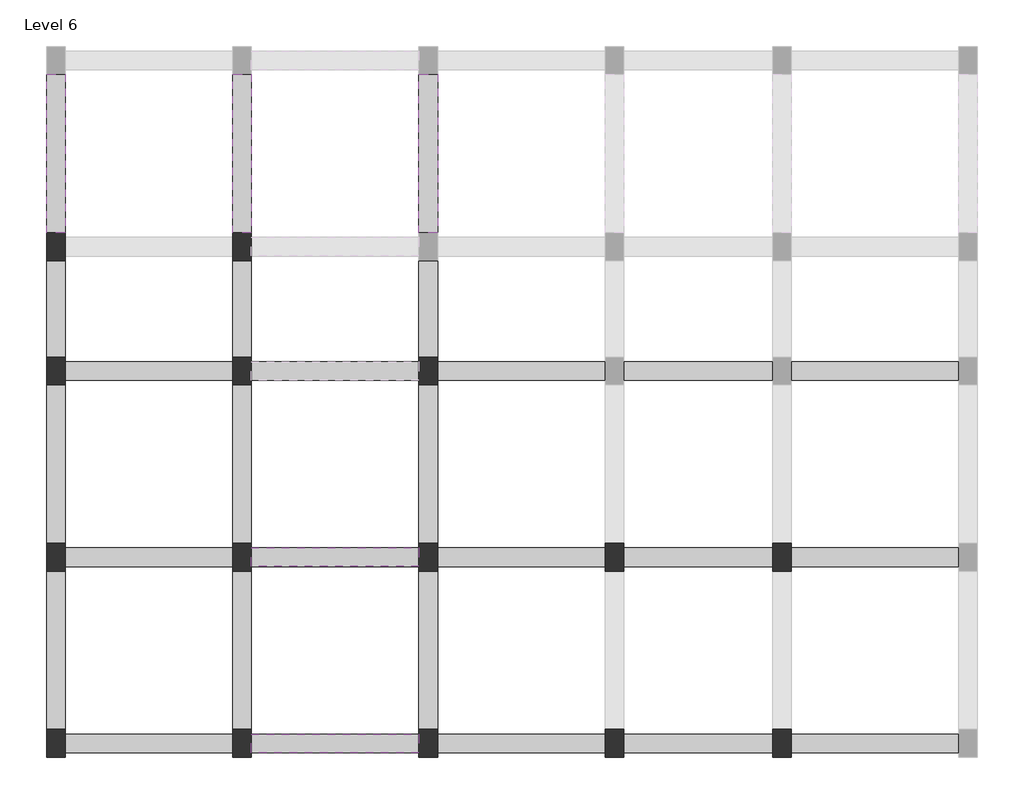
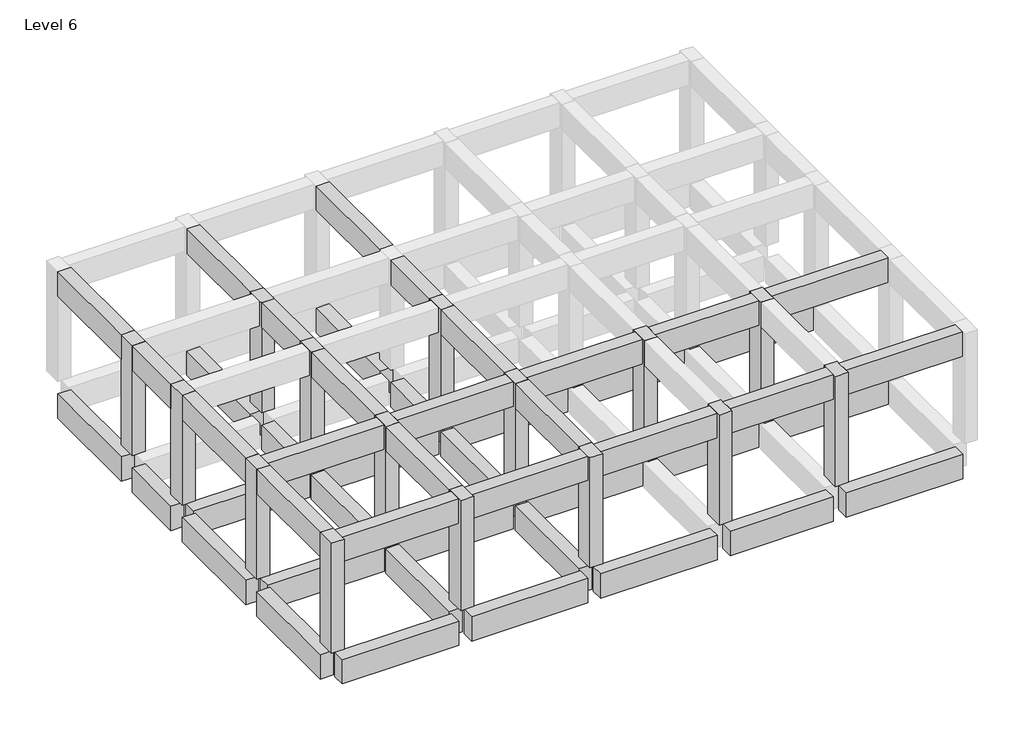
# One storey, part 1 of 2: 15 columns, 11 beams.
"""IFC4 building model written with IfcOpenShell, lengths in millimetres."""

from ifc_helpers import new_model, si_unit, frame, origin, place, context, project, spatial, polyline, outline, extrude, faceted_brep, element, save

model = new_model("IFC4")

# Units and contexts
model_context = context("Model", 3, world=origin())
ifc_project = project(units=[si_unit("LENGTHUNIT", "METRE", prefix="MILLI")], contexts=[model_context])

# Site, building, storey
site = spatial("IfcSite", under=ifc_project)
building = spatial("IfcBuilding", under=site)
storey = spatial("IfcBuildingStorey", under=building, Name="Level 6", Elevation=15240.0)

# Beams
placement = place(None, origin())
element("IfcBeam", 1, ObjectType="Concrete-Rectangular Beam : 12 x 24", at=placement, inside=storey, context=model_context, shape_type="SweptSolid", body=[
    extrude(outline(polyline([(2607.7603583, 7596.6647757), (2607.7603583, 7291.8647757), (-135.4396417, 7291.8647757), (-135.4396417, 7596.6647757), (2607.7603583, 7596.6647757)])), frame((0.0, 0.0, 14325.6), z_axis=(0.0, 0.0, 1.0), x_axis=(1.0, 0.0, 0.0)), (0.0, 0.0, 1.0), 609.6),
    extrude(outline(polyline([(-12022.6396417, 7291.8647757), (-12022.6396417, 7596.6647757), (-9279.4396417, 7596.6647757), (-9279.4396417, 7291.8647757), (-12022.6396417, 7291.8647757)])), frame((0.0, 0.0, 14325.6), z_axis=(0.0, 0.0, 1.0), x_axis=(1.0, 0.0, 0.0)), (0.0, 0.0, 1.0), 609.6),
    extrude(outline(polyline([(-8974.6396417, 7291.8647757), (-8974.6396417, 7596.6647757), (-6231.4396417, 7596.6647757), (-6231.4396417, 7291.8647757), (-8974.6396417, 7291.8647757)])), frame((0.0, 0.0, 14325.6), z_axis=(0.0, 0.0, 1.0), x_axis=(1.0, 0.0, 0.0)), (0.0, 0.0, 1.0), 609.6),
    extrude(outline(polyline([(-5926.6396417, 7291.8647757), (-5926.6396417, 7596.6647757), (-3183.4396417, 7596.6647757), (-3183.4396417, 7291.8647757), (-5926.6396417, 7291.8647757)])), frame((0.0, 0.0, 14325.6), z_axis=(0.0, 0.0, 1.0), x_axis=(1.0, 0.0, 0.0)), (0.0, 0.0, 1.0), 609.6),
    extrude(outline(polyline([(-2878.6396417, 7291.8647757), (-2878.6396417, 7596.6647757), (-440.2396417, 7596.6647757), (-440.2396417, 7291.8647757), (-2878.6396417, 7291.8647757)])), frame((0.0, 0.0, 14325.6), z_axis=(0.0, 0.0, 1.0), x_axis=(1.0, 0.0, 0.0)), (0.0, 0.0, 1.0), 609.6),
])
element("IfcBeam", 2, ObjectType="Concrete-Rectangular Beam : 12 x 24", at=placement, inside=storey, context=model_context, shape_type="SweptSolid", body=[
    extrude(outline(polyline([(2607.7603583, 10644.6647757), (2607.7603583, 10339.8647757), (-135.4396417, 10339.8647757), (-135.4396417, 10644.6647757), (2607.7603583, 10644.6647757)])), frame((0.0, 0.0, 14325.6), z_axis=(0.0, 0.0, 1.0), x_axis=(1.0, 0.0, 0.0)), (0.0, 0.0, 1.0), 609.6),
    extrude(outline(polyline([(-12022.6396417, 10339.8647757), (-12022.6396417, 10644.6647757), (-9279.4396417, 10644.6647757), (-9279.4396417, 10339.8647757), (-12022.6396417, 10339.8647757)])), frame((0.0, 0.0, 14325.6), z_axis=(0.0, 0.0, 1.0), x_axis=(1.0, 0.0, 0.0)), (0.0, 0.0, 1.0), 609.6),
    extrude(outline(polyline([(-8974.6396417, 10339.8647757), (-8974.6396417, 10644.6647757), (-6231.4396417, 10644.6647757), (-6231.4396417, 10339.8647757), (-8974.6396417, 10339.8647757)])), frame((0.0, 0.0, 14325.6), z_axis=(0.0, 0.0, 1.0), x_axis=(1.0, 0.0, 0.0)), (0.0, 0.0, 1.0), 609.6),
    extrude(outline(polyline([(-5926.6396417, 10339.8647757), (-5926.6396417, 10644.6647757), (-3183.4396417, 10644.6647757), (-3183.4396417, 10339.8647757), (-5926.6396417, 10339.8647757)])), frame((0.0, 0.0, 14325.6), z_axis=(0.0, 0.0, 1.0), x_axis=(1.0, 0.0, 0.0)), (0.0, 0.0, 1.0), 609.6),
    extrude(outline(polyline([(-2878.6396417, 10339.8647757), (-2878.6396417, 10644.6647757), (-440.2396417, 10644.6647757), (-440.2396417, 10339.8647757), (-2878.6396417, 10339.8647757)])), frame((0.0, 0.0, 14325.6), z_axis=(0.0, 0.0, 1.0), x_axis=(1.0, 0.0, 0.0)), (0.0, 0.0, 1.0), 609.6),
])
element("IfcBeam", 3, ObjectType="Concrete-Rectangular Beam : 12 x 24", at=placement, inside=storey, context=model_context, shape_type="SweptSolid", body=[
    extrude(outline(polyline([(2607.7603583, 13692.6647757), (2607.7603583, 13387.8647757), (-135.4396417, 13387.8647757), (-135.4396417, 13692.6647757), (2607.7603583, 13692.6647757)])), frame((0.0, 0.0, 14325.6), z_axis=(0.0, 0.0, 1.0), x_axis=(1.0, 0.0, 0.0)), (0.0, 0.0, 1.0), 609.6),
    extrude(outline(polyline([(-12022.6396417, 13387.8647757), (-12022.6396417, 13692.6647757), (-9279.4396417, 13692.6647757), (-9279.4396417, 13387.8647757), (-12022.6396417, 13387.8647757)])), frame((0.0, 0.0, 14325.6), z_axis=(0.0, 0.0, 1.0), x_axis=(1.0, 0.0, 0.0)), (0.0, 0.0, 1.0), 609.6),
    extrude(outline(polyline([(-8974.6396417, 13387.8647757), (-8974.6396417, 13692.6647757), (-6231.4396417, 13692.6647757), (-6231.4396417, 13387.8647757), (-8974.6396417, 13387.8647757)])), frame((0.0, 0.0, 14325.6), z_axis=(0.0, 0.0, 1.0), x_axis=(1.0, 0.0, 0.0)), (0.0, 0.0, 1.0), 609.6),
    extrude(outline(polyline([(-5926.6396417, 13387.8647757), (-5926.6396417, 13692.6647757), (-3183.4396417, 13692.6647757), (-3183.4396417, 13387.8647757), (-5926.6396417, 13387.8647757)])), frame((0.0, 0.0, 14325.6), z_axis=(0.0, 0.0, 1.0), x_axis=(1.0, 0.0, 0.0)), (0.0, 0.0, 1.0), 609.6),
    extrude(outline(polyline([(-2878.6396417, 13387.8647757), (-2878.6396417, 13692.6647757), (-440.2396417, 13692.6647757), (-440.2396417, 13387.8647757), (-2878.6396417, 13387.8647757)])), frame((0.0, 0.0, 14325.6), z_axis=(0.0, 0.0, 1.0), x_axis=(1.0, 0.0, 0.0)), (0.0, 0.0, 1.0), 609.6),
])
element("IfcBeam", 4, ObjectType="Concrete-Rectangular Beam : 12 x 24", at=placement, inside=storey, context=model_context, shape_type="SweptSolid", body=[
    extrude(outline(polyline([(-12022.6396417, 7672.8647757), (-12327.4396417, 7672.8647757), (-12327.4396417, 10263.6647757), (-12022.6396417, 10263.6647757), (-12022.6396417, 7672.8647757)])), frame((0.0, 0.0, 14325.6), z_axis=(0.0, 0.0, 1.0), x_axis=(1.0, 0.0, 0.0)), (0.0, 0.0, 1.0), 609.6),
    extrude(outline(polyline([(-12327.4396417, 18394.9119241), (-12022.6396417, 18394.9119241), (-12022.6396417, 15804.1119241), (-12327.4396417, 15804.1119241), (-12327.4396417, 18394.9119241)])), frame((0.0, 0.0, 14325.6), z_axis=(0.0, 0.0, 1.0), x_axis=(1.0, 0.0, 0.0)), (0.0, 0.0, 1.0), 609.6),
    extrude(outline(polyline([(-12022.6396417, 10720.8647757), (-12327.4396417, 10720.8647757), (-12327.4396417, 13311.6647757), (-12022.6396417, 13311.6647757), (-12022.6396417, 10720.8647757)])), frame((0.0, 0.0, 14325.6), z_axis=(0.0, 0.0, 1.0), x_axis=(1.0, 0.0, 0.0)), (0.0, 0.0, 1.0), 609.6),
    extrude(outline(polyline([(-12022.6396417, 13768.8647757), (-12327.4396417, 13768.8647757), (-12327.4396417, 15346.9119241), (-12022.6396417, 15346.9119241), (-12022.6396417, 13768.8647757)])), frame((0.0, 0.0, 14325.6), z_axis=(0.0, 0.0, 1.0), x_axis=(1.0, 0.0, 0.0)), (0.0, 0.0, 1.0), 609.6),
])
element("IfcBeam", 5, ObjectType="Concrete-Rectangular Beam : 12 x 24", at=placement, inside=storey, context=model_context, shape_type="SweptSolid", body=[
    extrude(outline(polyline([(-8974.6396417, 7672.8647757), (-9279.4396417, 7672.8647757), (-9279.4396417, 10263.6647757), (-8974.6396417, 10263.6647757), (-8974.6396417, 7672.8647757)])), frame((0.0, 0.0, 14325.6), z_axis=(0.0, 0.0, 1.0), x_axis=(1.0, 0.0, 0.0)), (0.0, 0.0, 1.0), 609.6),
    extrude(outline(polyline([(-9279.4396417, 18394.9119241), (-8974.6396417, 18394.9119241), (-8974.6396417, 15804.1119241), (-9279.4396417, 15804.1119241), (-9279.4396417, 18394.9119241)])), frame((0.0, 0.0, 14325.6), z_axis=(0.0, 0.0, 1.0), x_axis=(1.0, 0.0, 0.0)), (0.0, 0.0, 1.0), 609.6),
    extrude(outline(polyline([(-8974.6396417, 10720.8647757), (-9279.4396417, 10720.8647757), (-9279.4396417, 13311.6647757), (-8974.6396417, 13311.6647757), (-8974.6396417, 10720.8647757)])), frame((0.0, 0.0, 14325.6), z_axis=(0.0, 0.0, 1.0), x_axis=(1.0, 0.0, 0.0)), (0.0, 0.0, 1.0), 609.6),
    extrude(outline(polyline([(-8974.6396417, 13768.8647757), (-9279.4396417, 13768.8647757), (-9279.4396417, 15346.9119241), (-8974.6396417, 15346.9119241), (-8974.6396417, 13768.8647757)])), frame((0.0, 0.0, 14325.6), z_axis=(0.0, 0.0, 1.0), x_axis=(1.0, 0.0, 0.0)), (0.0, 0.0, 1.0), 609.6),
])
element("IfcBeam", 6, ObjectType="Concrete-Rectangular Beam : 12 x 24", at=placement, inside=storey, context=model_context, shape_type="SweptSolid", body=[
    extrude(outline(polyline([(-5926.6396417, 7672.8647757), (-6231.4396417, 7672.8647757), (-6231.4396417, 10263.6647757), (-5926.6396417, 10263.6647757), (-5926.6396417, 7672.8647757)])), frame((0.0, 0.0, 14325.6), z_axis=(0.0, 0.0, 1.0), x_axis=(1.0, 0.0, 0.0)), (0.0, 0.0, 1.0), 609.6),
    extrude(outline(polyline([(-6231.4396417, 18394.9119241), (-5926.6396417, 18394.9119241), (-5926.6396417, 15804.1119241), (-6231.4396417, 15804.1119241), (-6231.4396417, 18394.9119241)])), frame((0.0, 0.0, 14325.6), z_axis=(0.0, 0.0, 1.0), x_axis=(1.0, 0.0, 0.0)), (0.0, 0.0, 1.0), 609.6),
    extrude(outline(polyline([(-5926.6396417, 10720.8647757), (-6231.4396417, 10720.8647757), (-6231.4396417, 13311.6647757), (-5926.6396417, 13311.6647757), (-5926.6396417, 10720.8647757)])), frame((0.0, 0.0, 14325.6), z_axis=(0.0, 0.0, 1.0), x_axis=(1.0, 0.0, 0.0)), (0.0, 0.0, 1.0), 609.6),
    extrude(outline(polyline([(-5926.6396417, 13768.8647757), (-6231.4396417, 13768.8647757), (-6231.4396417, 15346.9119241), (-5926.6396417, 15346.9119241), (-5926.6396417, 13768.8647757)])), frame((0.0, 0.0, 14325.6), z_axis=(0.0, 0.0, 1.0), x_axis=(1.0, 0.0, 0.0)), (0.0, 0.0, 1.0), 609.6),
])
element("IfcBeam", 7, ObjectType="Concrete-Rectangular Beam : 12 x 24", at=placement, inside=storey, context=model_context, shape_type="SweptSolid", body=[
    extrude(outline(polyline([(2607.7603583, 7596.6647757), (2607.7603583, 7291.8647757), (-135.4396417, 7291.8647757), (-135.4396417, 7596.6647757), (2607.7603583, 7596.6647757)])), frame((0.0, 0.0, 17373.6), z_axis=(0.0, 0.0, 1.0), x_axis=(1.0, 0.0, 0.0)), (0.0, 0.0, 1.0), 609.6),
    extrude(outline(polyline([(-12022.6396417, 7291.8647757), (-12022.6396417, 7596.6647757), (-9279.4396417, 7596.6647757), (-9279.4396417, 7291.8647757), (-12022.6396417, 7291.8647757)])), frame((0.0, 0.0, 17373.6), z_axis=(0.0, 0.0, 1.0), x_axis=(1.0, 0.0, 0.0)), (0.0, 0.0, 1.0), 609.6),
    extrude(outline(polyline([(-8974.6396417, 7291.8647757), (-8974.6396417, 7596.6647757), (-6231.4396417, 7596.6647757), (-6231.4396417, 7291.8647757), (-8974.6396417, 7291.8647757)])), frame((0.0, 0.0, 17373.6), z_axis=(0.0, 0.0, 1.0), x_axis=(1.0, 0.0, 0.0)), (0.0, 0.0, 1.0), 609.6),
    extrude(outline(polyline([(-5926.6396417, 7291.8647757), (-5926.6396417, 7596.6647757), (-3183.4396417, 7596.6647757), (-3183.4396417, 7291.8647757), (-5926.6396417, 7291.8647757)])), frame((0.0, 0.0, 17373.6), z_axis=(0.0, 0.0, 1.0), x_axis=(1.0, 0.0, 0.0)), (0.0, 0.0, 1.0), 609.6),
    extrude(outline(polyline([(-2878.6396417, 7291.8647757), (-2878.6396417, 7596.6647757), (-440.2396417, 7596.6647757), (-440.2396417, 7291.8647757), (-2878.6396417, 7291.8647757)])), frame((0.0, 0.0, 17373.6), z_axis=(0.0, 0.0, 1.0), x_axis=(1.0, 0.0, 0.0)), (0.0, 0.0, 1.0), 609.6),
])
element("IfcBeam", 8, ObjectType="Concrete-Rectangular Beam : 12 x 24", at=placement, inside=storey, context=model_context, shape_type="SweptSolid", body=[
    extrude(outline(polyline([(2607.7603583, 10644.6647757), (2607.7603583, 10339.8647757), (-135.4396417, 10339.8647757), (-135.4396417, 10644.6647757), (2607.7603583, 10644.6647757)])), frame((0.0, 0.0, 17373.6), z_axis=(0.0, 0.0, 1.0), x_axis=(1.0, 0.0, 0.0)), (0.0, 0.0, 1.0), 609.6),
    extrude(outline(polyline([(-12022.6396417, 10339.8647757), (-12022.6396417, 10644.6647757), (-9279.4396417, 10644.6647757), (-9279.4396417, 10339.8647757), (-12022.6396417, 10339.8647757)])), frame((0.0, 0.0, 17373.6), z_axis=(0.0, 0.0, 1.0), x_axis=(1.0, 0.0, 0.0)), (0.0, 0.0, 1.0), 609.6),
    extrude(outline(polyline([(-8974.6396417, 10339.8647757), (-8974.6396417, 10644.6647757), (-6231.4396417, 10644.6647757), (-6231.4396417, 10339.8647757), (-8974.6396417, 10339.8647757)])), frame((0.0, 0.0, 17373.6), z_axis=(0.0, 0.0, 1.0), x_axis=(1.0, 0.0, 0.0)), (0.0, 0.0, 1.0), 609.6),
    extrude(outline(polyline([(-5926.6396417, 10339.8647757), (-5926.6396417, 10644.6647757), (-3183.4396417, 10644.6647757), (-3183.4396417, 10339.8647757), (-5926.6396417, 10339.8647757)])), frame((0.0, 0.0, 17373.6), z_axis=(0.0, 0.0, 1.0), x_axis=(1.0, 0.0, 0.0)), (0.0, 0.0, 1.0), 609.6),
    extrude(outline(polyline([(-2878.6396417, 10339.8647757), (-2878.6396417, 10644.6647757), (-440.2396417, 10644.6647757), (-440.2396417, 10339.8647757), (-2878.6396417, 10339.8647757)])), frame((0.0, 0.0, 17373.6), z_axis=(0.0, 0.0, 1.0), x_axis=(1.0, 0.0, 0.0)), (0.0, 0.0, 1.0), 609.6),
])
element("IfcBeam", 9, ObjectType="Concrete-Rectangular Beam : 12 x 24", at=placement, inside=storey, context=model_context, shape_type="SweptSolid", body=[
    extrude(outline(polyline([(-12022.6396417, 7672.8647757), (-12327.4396417, 7672.8647757), (-12327.4396417, 10263.6647757), (-12022.6396417, 10263.6647757), (-12022.6396417, 7672.8647757)])), frame((0.0, 0.0, 17373.6), z_axis=(0.0, 0.0, 1.0), x_axis=(1.0, 0.0, 0.0)), (0.0, 0.0, 1.0), 609.6),
    extrude(outline(polyline([(-12327.4396417, 18394.9119241), (-12022.6396417, 18394.9119241), (-12022.6396417, 15804.1119241), (-12327.4396417, 15804.1119241), (-12327.4396417, 18394.9119241)])), frame((0.0, 0.0, 17373.6), z_axis=(0.0, 0.0, 1.0), x_axis=(1.0, 0.0, 0.0)), (0.0, 0.0, 1.0), 609.6),
    extrude(outline(polyline([(-12022.6396417, 10720.8647757), (-12327.4396417, 10720.8647757), (-12327.4396417, 13311.6647757), (-12022.6396417, 13311.6647757), (-12022.6396417, 10720.8647757)])), frame((0.0, 0.0, 17373.6), z_axis=(0.0, 0.0, 1.0), x_axis=(1.0, 0.0, 0.0)), (0.0, 0.0, 1.0), 609.6),
    extrude(outline(polyline([(-12022.6396417, 13768.8647757), (-12327.4396417, 13768.8647757), (-12327.4396417, 15346.9119241), (-12022.6396417, 15346.9119241), (-12022.6396417, 13768.8647757)])), frame((0.0, 0.0, 17373.6), z_axis=(0.0, 0.0, 1.0), x_axis=(1.0, 0.0, 0.0)), (0.0, 0.0, 1.0), 609.6),
])
element("IfcBeam", 10, ObjectType="Concrete-Rectangular Beam : 12 x 24", at=placement, inside=storey, context=model_context, shape_type="SweptSolid", body=[
    extrude(outline(polyline([(-8974.6396417, 7672.8647757), (-9279.4396417, 7672.8647757), (-9279.4396417, 10263.6647757), (-8974.6396417, 10263.6647757), (-8974.6396417, 7672.8647757)])), frame((0.0, 0.0, 17373.6), z_axis=(0.0, 0.0, 1.0), x_axis=(1.0, 0.0, 0.0)), (0.0, 0.0, 1.0), 609.6),
    extrude(outline(polyline([(-9279.4396417, 18394.9119241), (-8974.6396417, 18394.9119241), (-8974.6396417, 15804.1119241), (-9279.4396417, 15804.1119241), (-9279.4396417, 18394.9119241)])), frame((0.0, 0.0, 17373.6), z_axis=(0.0, 0.0, 1.0), x_axis=(1.0, 0.0, 0.0)), (0.0, 0.0, 1.0), 609.6),
    extrude(outline(polyline([(-8974.6396417, 10720.8647757), (-9279.4396417, 10720.8647757), (-9279.4396417, 13311.6647757), (-8974.6396417, 13311.6647757), (-8974.6396417, 10720.8647757)])), frame((0.0, 0.0, 17373.6), z_axis=(0.0, 0.0, 1.0), x_axis=(1.0, 0.0, 0.0)), (0.0, 0.0, 1.0), 609.6),
    extrude(outline(polyline([(-8974.6396417, 13768.8647757), (-9279.4396417, 13768.8647757), (-9279.4396417, 15346.9119241), (-8974.6396417, 15346.9119241), (-8974.6396417, 13768.8647757)])), frame((0.0, 0.0, 17373.6), z_axis=(0.0, 0.0, 1.0), x_axis=(1.0, 0.0, 0.0)), (0.0, 0.0, 1.0), 609.6),
])
element("IfcBeam", 11, ObjectType="Concrete-Rectangular Beam : 12 x 24", at=placement, inside=storey, context=model_context, shape_type="SweptSolid", body=[
    extrude(outline(polyline([(-5926.6396417, 7672.8647757), (-6231.4396417, 7672.8647757), (-6231.4396417, 10263.6647757), (-5926.6396417, 10263.6647757), (-5926.6396417, 7672.8647757)])), frame((0.0, 0.0, 17373.6), z_axis=(0.0, 0.0, 1.0), x_axis=(1.0, 0.0, 0.0)), (0.0, 0.0, 1.0), 609.6),
    extrude(outline(polyline([(-6231.4396417, 18394.9119241), (-5926.6396417, 18394.9119241), (-5926.6396417, 15804.1119241), (-6231.4396417, 15804.1119241), (-6231.4396417, 18394.9119241)])), frame((0.0, 0.0, 17373.6), z_axis=(0.0, 0.0, 1.0), x_axis=(1.0, 0.0, 0.0)), (0.0, 0.0, 1.0), 609.6),
    extrude(outline(polyline([(-5926.6396417, 10720.8647757), (-6231.4396417, 10720.8647757), (-6231.4396417, 13311.6647757), (-5926.6396417, 13311.6647757), (-5926.6396417, 10720.8647757)])), frame((0.0, 0.0, 17373.6), z_axis=(0.0, 0.0, 1.0), x_axis=(1.0, 0.0, 0.0)), (0.0, 0.0, 1.0), 609.6),
    extrude(outline(polyline([(-5926.6396417, 13768.8647757), (-6231.4396417, 13768.8647757), (-6231.4396417, 15346.9119241), (-5926.6396417, 15346.9119241), (-5926.6396417, 13768.8647757)])), frame((0.0, 0.0, 17373.6), z_axis=(0.0, 0.0, 1.0), x_axis=(1.0, 0.0, 0.0)), (0.0, 0.0, 1.0), 609.6),
])

# Columns
element("IfcColumn", 12, ObjectType="Concrete-Rectangular-Column : c1", at=placement, inside=storey, context=model_context, shape_type="SweptSolid", body=[
    extrude(outline(polyline([(-12327.4396417, 7215.6647757), (-12327.4396417, 7672.8647757), (-12022.6396417, 7672.8647757), (-12022.6396417, 7215.6647757), (-12327.4396417, 7215.6647757)])), frame((0.0, 0.0, 15240.0), z_axis=(0.0, 0.0, 1.0), x_axis=(1.0, 0.0, 0.0)), (0.0, 0.0, 1.0), 2743.2),
])
element("IfcColumn", 13, ObjectType="Concrete-Rectangular-Column : c1", at=placement, inside=storey, context=model_context, shape_type="Brep", body=[
    faceted_brep([(-9279.4396417, 7215.6647757, 15240.0), (-9279.4396417, 7672.8647757, 15240.0), (-8974.6396417, 7672.8647757, 15240.0), (-8974.6396417, 7215.6647757, 15240.0), (-9279.4396417, 7215.6647757, 17983.2), (-9279.4396417, 7291.8647757, 17983.2), (-9279.4396417, 7596.6647757, 17983.2), (-9279.4396417, 7672.8647757, 17983.2), (-8974.6396417, 7672.8647757, 17983.2), (-8974.6396417, 7596.6647757, 17983.2), (-8974.6396417, 7291.8647757, 17983.2), (-8974.6396417, 7215.6647757, 17983.2)], [[[0, 1, 2, 3]], [[4, 5, 6, 7, 1, 0]], [[7, 8, 2, 1]], [[8, 9, 10, 11, 3, 2]], [[11, 4, 0, 3]], [[4, 11, 10, 9, 8, 7, 6, 5]]]),
])
element("IfcColumn", 14, ObjectType="Concrete-Rectangular-Column : c1", at=placement, inside=storey, context=model_context, shape_type="Brep", body=[
    faceted_brep([(-6231.4396417, 7215.6647757, 15240.0), (-6231.4396417, 7672.8647757, 15240.0), (-5926.6396417, 7672.8647757, 15240.0), (-5926.6396417, 7215.6647757, 15240.0), (-6231.4396417, 7215.6647757, 17983.2), (-6231.4396417, 7291.8647757, 17983.2), (-6231.4396417, 7596.6647757, 17983.2), (-6231.4396417, 7672.8647757, 17983.2), (-5926.6396417, 7672.8647757, 17983.2), (-5926.6396417, 7596.6647757, 17983.2), (-5926.6396417, 7291.8647757, 17983.2), (-5926.6396417, 7215.6647757, 17983.2)], [[[0, 1, 2, 3]], [[4, 5, 6, 7, 1, 0]], [[7, 8, 2, 1]], [[8, 9, 10, 11, 3, 2]], [[11, 4, 0, 3]], [[4, 11, 10, 9, 8, 7, 6, 5]]]),
])
element("IfcColumn", 15, ObjectType="Concrete-Rectangular-Column : c1", at=placement, inside=storey, context=model_context, shape_type="Brep", body=[
    faceted_brep([(-3183.4396417, 7215.6647757, 15240.0), (-3183.4396417, 7672.8647757, 15240.0), (-2878.6396417, 7672.8647757, 15240.0), (-2878.6396417, 7215.6647757, 15240.0), (-3183.4396417, 7215.6647757, 17983.2), (-3183.4396417, 7291.8647757, 17983.2), (-3183.4396417, 7596.6647757, 17983.2), (-3183.4396417, 7672.8647757, 17983.2), (-2878.6396417, 7672.8647757, 17983.2), (-2878.6396417, 7596.6647757, 17983.2), (-2878.6396417, 7291.8647757, 17983.2), (-2878.6396417, 7215.6647757, 17983.2)], [[[0, 1, 2, 3]], [[4, 5, 6, 7, 1, 0]], [[7, 8, 2, 1]], [[8, 9, 10, 11, 3, 2]], [[11, 4, 0, 3]], [[4, 11, 10, 9, 8, 7, 6, 5]]]),
])
element("IfcColumn", 16, ObjectType="Concrete-Rectangular-Column : c1", at=placement, inside=storey, context=model_context, shape_type="Brep", body=[
    faceted_brep([(-440.2396417, 7215.6647757, 15240.0), (-440.2396417, 7672.8647757, 15240.0), (-135.4396417, 7672.8647757, 15240.0), (-135.4396417, 7215.6647757, 15240.0), (-440.2396417, 7215.6647757, 17983.2), (-440.2396417, 7291.8647757, 17983.2), (-440.2396417, 7596.6647757, 17983.2), (-440.2396417, 7672.8647757, 17983.2), (-135.4396417, 7672.8647757, 17983.2), (-135.4396417, 7596.6647757, 17983.2), (-135.4396417, 7291.8647757, 17983.2), (-135.4396417, 7215.6647757, 17983.2)], [[[0, 1, 2, 3]], [[4, 5, 6, 7, 1, 0]], [[7, 8, 2, 1]], [[8, 9, 10, 11, 3, 2]], [[11, 4, 0, 3]], [[4, 11, 10, 9, 8, 7, 6, 5]]]),
])
element("IfcColumn", 17, ObjectType="Concrete-Rectangular-Column : c1", at=placement, inside=storey, context=model_context, shape_type="Brep", body=[
    faceted_brep([(-12327.4396417, 10263.6647757, 15240.0), (-12327.4396417, 10720.8647757, 15240.0), (-12022.6396417, 10720.8647757, 15240.0), (-12022.6396417, 10263.6647757, 15240.0), (-12327.4396417, 10263.6647757, 17983.2), (-12327.4396417, 10720.8647757, 17983.2), (-12327.4396417, 10720.8647757, 17373.6), (-12327.4396417, 10263.6647757, 17373.6), (-12022.6396417, 10720.8647757, 17983.2), (-12022.6396417, 10720.8647757, 17373.6), (-12022.6396417, 10263.6647757, 17983.2), (-12022.6396417, 10263.6647757, 17373.6)], [[[0, 1, 2, 3]], [[4, 5, 6, 1, 0, 7]], [[5, 8, 9, 2, 1, 6]], [[8, 10, 11, 3, 2, 9]], [[10, 4, 7, 0, 3, 11]], [[4, 10, 8, 5]]]),
])
element("IfcColumn", 18, ObjectType="Concrete-Rectangular-Column : c1", at=placement, inside=storey, context=model_context, shape_type="Brep", body=[
    faceted_brep([(-9279.4396417, 10263.6647757, 15240.0), (-9279.4396417, 10720.8647757, 15240.0), (-8974.6396417, 10720.8647757, 15240.0), (-8974.6396417, 10263.6647757, 15240.0), (-9279.4396417, 10263.6647757, 17983.2), (-9279.4396417, 10339.8647757, 17983.2), (-9279.4396417, 10644.6647757, 17983.2), (-9279.4396417, 10720.8647757, 17983.2), (-9279.4396417, 10720.8647757, 17373.6), (-9279.4396417, 10263.6647757, 17373.6), (-8974.6396417, 10720.8647757, 17983.2), (-8974.6396417, 10720.8647757, 17373.6), (-8974.6396417, 10644.6647757, 17983.2), (-8974.6396417, 10339.8647757, 17983.2), (-8974.6396417, 10263.6647757, 17983.2), (-8974.6396417, 10263.6647757, 17373.6)], [[[0, 1, 2, 3]], [[4, 5, 6, 7, 8, 1, 0, 9]], [[7, 10, 11, 2, 1, 8]], [[10, 12, 13, 14, 15, 3, 2, 11]], [[14, 4, 9, 0, 3, 15]], [[4, 14, 13, 12, 10, 7, 6, 5]]]),
])
element("IfcColumn", 19, ObjectType="Concrete-Rectangular-Column : c1", at=placement, inside=storey, context=model_context, shape_type="Brep", body=[
    faceted_brep([(-6231.4396417, 10263.6647757, 15240.0), (-6231.4396417, 10720.8647757, 15240.0), (-5926.6396417, 10720.8647757, 15240.0), (-5926.6396417, 10263.6647757, 15240.0), (-6231.4396417, 10263.6647757, 17983.2), (-6231.4396417, 10339.8647757, 17983.2), (-6231.4396417, 10644.6647757, 17983.2), (-6231.4396417, 10720.8647757, 17983.2), (-6231.4396417, 10720.8647757, 17373.6), (-6231.4396417, 10263.6647757, 17373.6), (-5926.6396417, 10720.8647757, 17983.2), (-5926.6396417, 10720.8647757, 17373.6), (-5926.6396417, 10644.6647757, 17983.2), (-5926.6396417, 10339.8647757, 17983.2), (-5926.6396417, 10263.6647757, 17983.2), (-5926.6396417, 10263.6647757, 17373.6)], [[[0, 1, 2, 3]], [[4, 5, 6, 7, 8, 1, 0, 9]], [[7, 10, 11, 2, 1, 8]], [[10, 12, 13, 14, 15, 3, 2, 11]], [[14, 4, 9, 0, 3, 15]], [[4, 14, 13, 12, 10, 7, 6, 5]]]),
])
element("IfcColumn", 20, ObjectType="Concrete-Rectangular-Column : c1", at=placement, inside=storey, context=model_context, shape_type="Brep", body=[
    faceted_brep([(-3183.4396417, 10263.6647757, 15240.0), (-3183.4396417, 10720.8647757, 15240.0), (-2878.6396417, 10720.8647757, 15240.0), (-2878.6396417, 10263.6647757, 15240.0), (-3183.4396417, 10263.6647757, 17983.2), (-3183.4396417, 10339.8647757, 17983.2), (-3183.4396417, 10644.6647757, 17983.2), (-3183.4396417, 10720.8647757, 17983.2), (-3183.4396417, 10720.8647757, 17373.6), (-3183.4396417, 10263.6647757, 17373.6), (-2878.6396417, 10720.8647757, 17983.2), (-2878.6396417, 10720.8647757, 17373.6), (-2878.6396417, 10644.6647757, 17983.2), (-2878.6396417, 10339.8647757, 17983.2), (-2878.6396417, 10263.6647757, 17983.2), (-2878.6396417, 10263.6647757, 17373.6)], [[[0, 1, 2, 3]], [[4, 5, 6, 7, 8, 1, 0, 9]], [[7, 10, 11, 2, 1, 8]], [[10, 12, 13, 14, 15, 3, 2, 11]], [[14, 4, 9, 0, 3, 15]], [[4, 14, 13, 12, 10, 7, 6, 5]]]),
])
element("IfcColumn", 21, ObjectType="Concrete-Rectangular-Column : c1", at=placement, inside=storey, context=model_context, shape_type="Brep", body=[
    faceted_brep([(-440.2396417, 10263.6647757, 15240.0), (-440.2396417, 10720.8647757, 15240.0), (-135.4396417, 10720.8647757, 15240.0), (-135.4396417, 10263.6647757, 15240.0), (-440.2396417, 10263.6647757, 17983.2), (-440.2396417, 10339.8647757, 17983.2), (-440.2396417, 10644.6647757, 17983.2), (-440.2396417, 10720.8647757, 17983.2), (-440.2396417, 10720.8647757, 17373.6), (-440.2396417, 10263.6647757, 17373.6), (-135.4396417, 10720.8647757, 17983.2), (-135.4396417, 10720.8647757, 17373.6), (-135.4396417, 10644.6647757, 17983.2), (-135.4396417, 10339.8647757, 17983.2), (-135.4396417, 10263.6647757, 17983.2), (-135.4396417, 10263.6647757, 17373.6)], [[[0, 1, 2, 3]], [[4, 5, 6, 7, 8, 1, 0, 9]], [[7, 10, 11, 2, 1, 8]], [[10, 12, 13, 14, 15, 3, 2, 11]], [[14, 4, 9, 0, 3, 15]], [[4, 14, 13, 12, 10, 7, 6, 5]]]),
])
element("IfcColumn", 22, ObjectType="Concrete-Rectangular-Column : c1", at=placement, inside=storey, context=model_context, shape_type="Brep", body=[
    faceted_brep([(-12327.4396417, 13311.6647757, 15240.0), (-12327.4396417, 13768.8647757, 15240.0), (-12022.6396417, 13768.8647757, 15240.0), (-12022.6396417, 13311.6647757, 15240.0), (-12327.4396417, 13311.6647757, 17983.2), (-12327.4396417, 13768.8647757, 17983.2), (-12327.4396417, 13768.8647757, 17373.6), (-12327.4396417, 13311.6647757, 17373.6), (-12022.6396417, 13768.8647757, 17983.2), (-12022.6396417, 13768.8647757, 17373.6), (-12022.6396417, 13311.6647757, 17983.2), (-12022.6396417, 13311.6647757, 17373.6)], [[[0, 1, 2, 3]], [[4, 5, 6, 1, 0, 7]], [[5, 8, 9, 2, 1, 6]], [[8, 10, 11, 3, 2, 9]], [[10, 4, 7, 0, 3, 11]], [[4, 10, 8, 5]]]),
])
element("IfcColumn", 23, ObjectType="Concrete-Rectangular-Column : c1", at=placement, inside=storey, context=model_context, shape_type="Brep", body=[
    faceted_brep([(-9279.4396417, 13311.6647757, 15240.0), (-9279.4396417, 13768.8647757, 15240.0), (-8974.6396417, 13768.8647757, 15240.0), (-8974.6396417, 13311.6647757, 15240.0), (-9279.4396417, 13311.6647757, 17983.2), (-9279.4396417, 13387.8647757, 17983.2), (-9279.4396417, 13692.6647757, 17983.2), (-9279.4396417, 13768.8647757, 17983.2), (-9279.4396417, 13768.8647757, 17373.6), (-9279.4396417, 13311.6647757, 17373.6), (-8974.6396417, 13768.8647757, 17983.2), (-8974.6396417, 13768.8647757, 17373.6), (-8974.6396417, 13692.6647757, 17983.2), (-8974.6396417, 13387.8647757, 17983.2), (-8974.6396417, 13311.6647757, 17983.2), (-8974.6396417, 13311.6647757, 17373.6)], [[[0, 1, 2, 3]], [[4, 5, 6, 7, 8, 1, 0, 9]], [[7, 10, 11, 2, 1, 8]], [[10, 12, 13, 14, 15, 3, 2, 11]], [[14, 4, 9, 0, 3, 15]], [[4, 14, 13, 12, 10, 7, 6, 5]]]),
])
element("IfcColumn", 24, ObjectType="Concrete-Rectangular-Column : c1", at=placement, inside=storey, context=model_context, shape_type="Brep", body=[
    faceted_brep([(-6231.4396417, 13311.6647757, 15240.0), (-6231.4396417, 13768.8647757, 15240.0), (-5926.6396417, 13768.8647757, 15240.0), (-5926.6396417, 13311.6647757, 15240.0), (-6231.4396417, 13311.6647757, 17983.2), (-6231.4396417, 13387.8647757, 17983.2), (-6231.4396417, 13692.6647757, 17983.2), (-6231.4396417, 13768.8647757, 17983.2), (-6231.4396417, 13768.8647757, 17373.6), (-6231.4396417, 13311.6647757, 17373.6), (-5926.6396417, 13768.8647757, 17983.2), (-5926.6396417, 13768.8647757, 17373.6), (-5926.6396417, 13692.6647757, 17983.2), (-5926.6396417, 13387.8647757, 17983.2), (-5926.6396417, 13311.6647757, 17983.2), (-5926.6396417, 13311.6647757, 17373.6)], [[[0, 1, 2, 3]], [[4, 5, 6, 7, 8, 1, 0, 9]], [[7, 10, 11, 2, 1, 8]], [[10, 12, 13, 14, 15, 3, 2, 11]], [[14, 4, 9, 0, 3, 15]], [[4, 14, 13, 12, 10, 7, 6, 5]]]),
])
element("IfcColumn", 25, ObjectType="Concrete-Rectangular-Column : c1", at=placement, inside=storey, context=model_context, shape_type="Brep", body=[
    faceted_brep([(-12327.4396417, 15346.9119241, 15240.0), (-12327.4396417, 15804.1119241, 15240.0), (-12022.6396417, 15804.1119241, 15240.0), (-12022.6396417, 15346.9119241, 15240.0), (-12327.4396417, 15346.9119241, 17983.2), (-12327.4396417, 15804.1119241, 17983.2), (-12327.4396417, 15804.1119241, 17373.6), (-12327.4396417, 15346.9119241, 17373.6), (-12022.6396417, 15804.1119241, 17983.2), (-12022.6396417, 15804.1119241, 17373.6), (-12022.6396417, 15346.9119241, 17983.2), (-12022.6396417, 15346.9119241, 17373.6)], [[[0, 1, 2, 3]], [[4, 5, 6, 1, 0, 7]], [[5, 8, 9, 2, 1, 6]], [[8, 10, 11, 3, 2, 9]], [[10, 4, 7, 0, 3, 11]], [[4, 10, 8, 5]]]),
])
element("IfcColumn", 26, ObjectType="Concrete-Rectangular-Column : c1", at=placement, inside=storey, context=model_context, shape_type="Brep", body=[
    faceted_brep([(-9279.4396417, 15346.9119241, 15240.0), (-9279.4396417, 15804.1119241, 15240.0), (-8974.6396417, 15804.1119241, 15240.0), (-8974.6396417, 15346.9119241, 15240.0), (-9279.4396417, 15346.9119241, 17983.2), (-9279.4396417, 15423.1119241, 17983.2), (-9279.4396417, 15727.9119241, 17983.2), (-9279.4396417, 15804.1119241, 17983.2), (-9279.4396417, 15804.1119241, 17373.6), (-9279.4396417, 15346.9119241, 17373.6), (-8974.6396417, 15804.1119241, 17983.2), (-8974.6396417, 15804.1119241, 17373.6), (-8974.6396417, 15727.9119241, 17983.2), (-8974.6396417, 15423.1119241, 17983.2), (-8974.6396417, 15346.9119241, 17983.2), (-8974.6396417, 15346.9119241, 17373.6)], [[[0, 1, 2, 3]], [[4, 5, 6, 7, 8, 1, 0, 9]], [[7, 10, 11, 2, 1, 8]], [[10, 12, 13, 14, 15, 3, 2, 11]], [[14, 4, 9, 0, 3, 15]], [[4, 14, 13, 12, 10, 7, 6, 5]]]),
])

save(model, "model.ifc")

# Revit data of these elements
# Type "Concrete-Rectangular Beam : 12 x 24"
#   Assembly Code = "B10"
#   Length [instance default] = 5' - 0"
#   b = 1' - 0"
#   h = 2' - 0"
#   Structural Material [instance default] = Concrete, Cast-in-Place gray
# Type "Concrete-Rectangular-Column : c1"
#   Assembly Code = "B10"
#   b = 1' - 0"
#   h = 1' - 6"
#   Structural Material [instance default] = Concrete, Cast-in-Place gray
# Elements 1, 2, 3, 4, 5, 6, 7, 8, 9, 10, 11 (IfcBeam, "Concrete-Rectangular Beam : 12 x 24")
#   Structural Material = Concrete, Cast-in-Place gray
#   Phase Created = New Construction
#   Materials on its faces: "Concrete, Cast-in-Place gray"
# Elements 12, 13, 14, 15, 16, 17, 18, 19, 20, 21, 22, 23, 24, 25, 26 (IfcColumn, "Concrete-Rectangular-Column : c1")
#   Comments = ""
#   Structural Material = Concrete, Cast-in-Place gray
#   Phase Created = New Construction
#   Materials on its faces: "Concrete, Cast-in-Place gray"
# Materials
#   "Concrete, Cast-in-Place gray": class "Concrete", colour RGB 192 192 192, transparency 0, Description = "Cast-in-place concrete", Cost = 0
